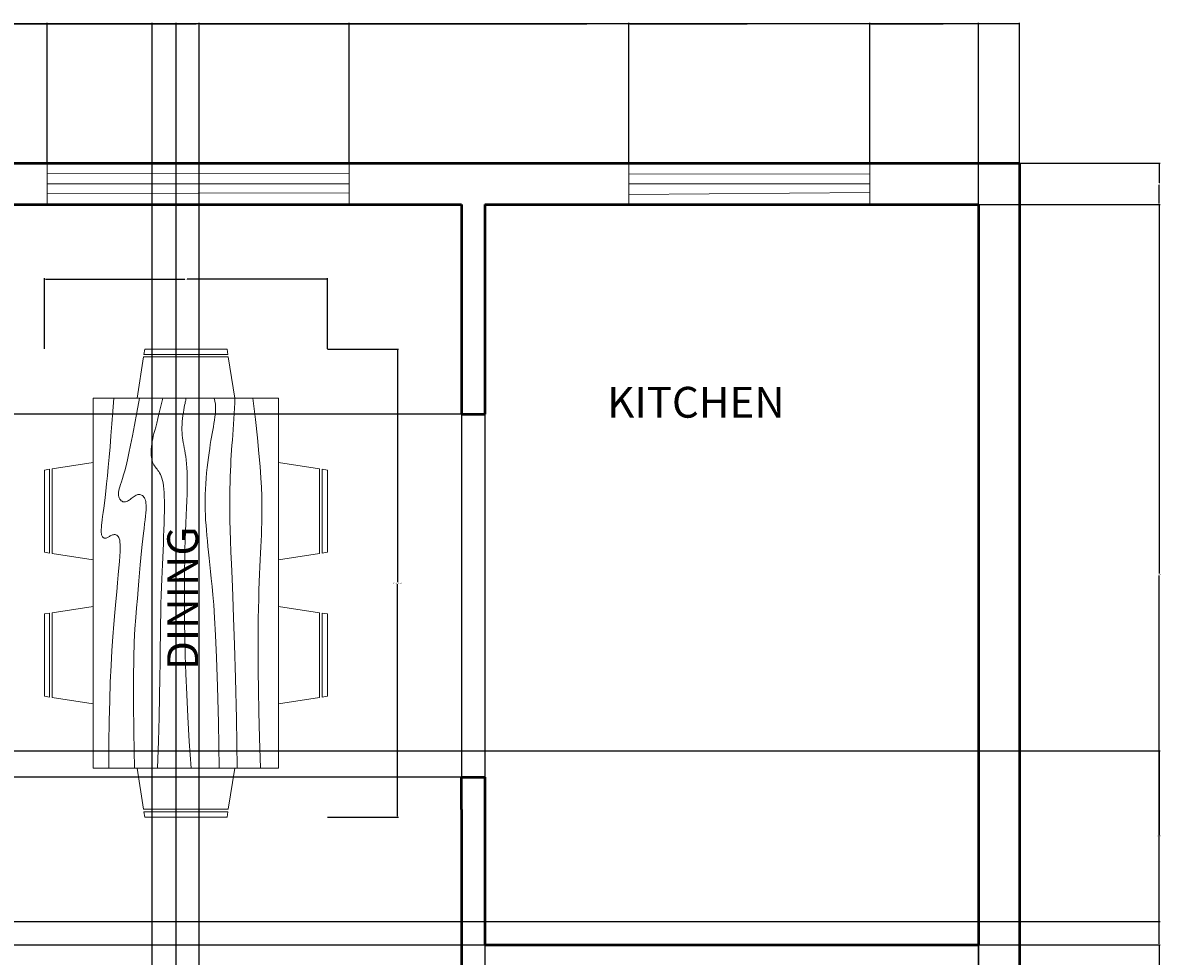
# Model space of a CAD drawing. Units: inches. Extents: x 2907 to 3328, y 1715 to 2286.
# Tile 5 of 5: x 3107 to 3328, y 2105 to 2286. Entities that reach past the tile are written whole.
import ezdxf

# ---------------------------------------------------------------- set-up
doc = ezdxf.new("R2010")
doc.units = ezdxf.units.IN
for name, color, linetype, lineweight in [('A-ANNO-DIMS', 2, 'Continuous', 18), ('A-AREA-IDEN', 7, 'Continuous', 25), ('A-FURN', 8, 'Continuous', 18), ('A-GLAZ', 4, 'Continuous', 18), ('A-WALL', 7, 'Continuous', 50)]:
    doc.layers.add(name, color=color, linetype=linetype, lineweight=lineweight)
doc.styles.get("Standard").update_dxf_attribs({"font": 'arial.ttf'})
doc.dimstyles.get("Standard").update_dxf_attribs({"dimtxt": 0.18, "dimasz": 0.18, "dimexe": 0.18, "dimexo": 0.0625, "dimgap": 0.09, "dimtad": 0, "dimtih": 1, "dimtoh": 1, "dimdec": 4, "dimzin": 0, "dimdsep": 46, "dimtxsty": 'Standard', "dimcen": 0.09, "dimadec": 0, "dimazin": 0, "dimtfac": 1, "dimtdec": 4, "dimtofl": 0, "dimtmove": 0, "dimatfit": 3, "dimfxl": 1, "dimtolj": 1, "dimtzin": 0, "dimarcsym": 0})

# ---------------------------------------------------------------- blocks, each defined once
blk = doc.blocks.new('Dining Set - 36 x 72 in.')
for p, q in [((-22, 27.5), (-22.1562, 26.50042)), ((-22, 27.5), (-6, 27.5)), ((-5.8437, 26.49966), (-6, 27.5)), ((6, 27.5), (5.8438, 26.50042)), ((6, 27.5), (22, 27.5)), ((22.1563, 26.49966), (22, 27.5)), ((-22.2343, 26.00059), (-23.4847, 17.99762)), ((-22.2304, 26), (-5.7608, 26)), ((-5.8416, 26.5), (-22.1534, 26.5)), ((-4.5152, 17.99762), (-5.7655, 25.99926)), ((5.7657, 26.00059), (4.5153, 17.99762)), ((5.7696, 26), (22.2392, 26)), ((22.1584, 26.5), (5.8466, 26.5)), ((23.4848, 17.99762), (22.2345, 25.99926)), ((36, 18), (-36, 18)), ((-36, 18), (-36, -18)), ((36, -18), (36, 18)), ((-44.0006, 8.23428), (-35.9976, 9.48474)), ((44.0006, 8.23428), (35.9976, 9.48474)), ((-45.5, 8), (-44.5004, 8.15617)), ((-45.5, 8), (-45.5, -8)), ((-44.5, -8.15843), (-44.5, 8.15338)), ((-44, 8.23041), (-44, -8.23915)), ((44, 8.23041), (44, -8.23915)), ((44.5, -8.15843), (44.5, 8.15338)), ((45.5, 8), (44.5005, 8.15617)), ((45.5, 8), (45.5, -8)), ((-44.4997, -8.15631), (-45.5, -8)), ((-35.9976, -9.48476), (-43.9993, -8.2345)), ((35.9976, -9.48476), (43.9993, -8.2345)), ((44.4997, -8.15631), (45.5, -8)), ((-36, -18), (36, -18)), ((-22.2343, -26.0006), (-23.4847, -17.99762)), ((-4.5152, -17.99762), (-5.7655, -25.99928)), ((5.7657, -26.0006), (4.5153, -17.99762)), ((23.4848, -17.99762), (22.2345, -25.99928)), ((-22.2304, -26), (-5.7608, -26)), ((-22, -27.5), (-22.1562, -26.50044)), ((-5.8416, -26.5), (-22.1534, -26.5)), ((-5.8437, -26.49967), (-6, -27.5)), ((5.7696, -26), (22.2392, -26)), ((6, -27.5), (5.8438, -26.50044)), ((22.1584, -26.5), (5.8466, -26.5)), ((22.1563, -26.49967), (22, -27.5)), ((-22, -27.5), (-6, -27.5)), ((6, -27.5), (22, -27.5))]:
    blk.add_line(p, q)
for points in [[(-36, 15), (-31.1772, 14.97754), (-26.8079, 14.91406), (-22.8538, 14.81543), (-19.276, 14.6875), (-16.0362, 14.53613), (-13.0957, 14.36718), (-10.4159, 14.18652), (-7.9583, 14), (-5.6904, 13.81315), (-3.6035, 13.63021), (-1.6954, 13.45508), (0.0365, 13.29166), (1.5945, 13.14388), (2.9811, 13.01562), (4.1988, 12.9108), (5.25, 12.83333), (6.1393, 12.78613), (6.8802, 12.76823), (7.4883, 12.77767), (7.9792, 12.8125), (8.3685, 12.87077), (8.6719, 12.95052), (8.9049, 13.0498), (9.0833, 13.16666), (9.2205, 13.29899), (9.3216, 13.44401), (9.3895, 13.59879), (9.4271, 13.76041), (9.4373, 13.92594), (9.4232, 14.09245), (9.3875, 14.257), (9.3333, 14.41666), (9.2638, 14.56917), (9.1836, 14.71484), (9.0975, 14.85465), (9.0104, 14.98958), (8.9272, 15.1206), (8.8529, 15.2487), (8.7922, 15.37483), (8.75, 15.5), (8.7305, 15.62467), (8.7344, 15.74739), (8.7617, 15.86621), (8.8125, 15.97916), (8.8867, 16.08431), (8.9844, 16.17968), (9.1055, 16.26334), (9.25, 16.33333), (9.4189, 16.38802), (9.6172, 16.42708), (9.8506, 16.45052), (10.125, 16.45833), (10.4463, 16.45052), (10.8203, 16.42708), (11.2529, 16.38802), (11.75, 16.33333), (12.3184, 16.26318), (12.9694, 16.17838), (13.7151, 16.07991), (14.5677, 15.96875), (15.5395, 15.84586), (16.6426, 15.71224), (17.8893, 15.56884), (19.2917, 15.41666), (20.859, 15.25667), (22.5879, 15.08984), (24.4721, 14.91715), (26.5052, 14.73958), (28.6809, 14.5581), (30.9929, 14.3737), (33.4347, 14.18733), (36, 14)], [(-36, 10), (-28.9766, 10.14274), (-23.1725, 10.20442), (-18.4241, 10.19775), (-14.5677, 10.13541), (-11.4399, 10.03011), (-8.877, 9.89453), (-6.7154, 9.74137), (-4.7917, 9.58333), (-2.9698, 9.43082), (-1.2246, 9.28515), (0.4415, 9.14534), (2.026, 9.01041), (3.5266, 8.87939), (4.9408, 8.7513), (6.266, 8.62516), (7.5, 8.5), (8.6411, 8.37549), (9.6914, 8.2539), (10.6538, 8.13818), (11.5312, 8.03125), (12.3267, 7.93603), (13.043, 7.85547), (13.6831, 7.79248), (14.25, 7.75), (14.7471, 7.7303), (15.1797, 7.73307), (15.5537, 7.75732), (15.875, 7.80208), (16.1494, 7.86637), (16.3828, 7.94922), (16.5811, 8.04964), (16.75, 8.16666), (16.8944, 8.29915), (17.0143, 8.44531), (17.1089, 8.60319), (17.1771, 8.77083), (17.218, 8.94629), (17.2305, 9.1276), (17.2137, 9.31282), (17.1667, 9.5), (17.0895, 9.6875), (16.987, 9.875), (16.8649, 10.0625), (16.7292, 10.25), (16.5856, 10.4375), (16.4401, 10.625), (16.2985, 10.8125), (16.1667, 11), (16.05, 11.18733), (15.9518, 11.3737), (15.8752, 11.5581), (15.8229, 11.73958), (15.798, 11.91715), (15.8034, 12.08984), (15.842, 12.25667), (15.9167, 12.41666), (16.0295, 12.56836), (16.1784, 12.70833), (16.3605, 12.83268), (16.5729, 12.9375), (16.8127, 13.01888), (17.0768, 13.07291), (17.3625, 13.0957), (17.6667, 13.08333), (17.9894, 13.03312), (18.3418, 12.94726), (18.7382, 12.82918), (19.1927, 12.68229), (19.7195, 12.51001), (20.3327, 12.31575), (21.0465, 12.10294), (21.875, 11.875), (22.8357, 11.63354), (23.959, 11.37304), (25.2786, 11.08618), (26.8282, 10.76562), (28.6414, 10.40405), (30.752, 9.99414), (33.1936, 9.52856), (36, 9)], [(-36, 5.5), (-30.7157, 5.3348), (-26.069, 5.20963), (-21.9946, 5.11767), (-18.4271, 5.05208), (-15.3009, 5.00602), (-12.5508, 4.97265), (-10.1112, 4.94515), (-7.9167, 4.91666), (-5.909, 4.88167), (-4.0586, 4.83984), (-2.3429, 4.79215), (-0.7396, 4.73958), (0.7739, 4.6831), (2.22, 4.6237), (3.6213, 4.56233), (5, 4.5), (6.373, 4.43782), (7.7344, 4.3776), (9.0723, 4.32129), (10.375, 4.27083), (11.6309, 4.22819), (12.8281, 4.19531), (13.9551, 4.17415), (15, 4.16666), (15.954, 4.17448), (16.819, 4.19791), (17.6001, 4.23698), (18.3021, 4.29166), (18.9299, 4.36198), (19.4883, 4.44791), (19.9823, 4.54948), (20.4167, 4.66666), (20.7969, 4.79899), (21.1302, 4.94401), (21.4245, 5.09879), (21.6875, 5.26041), (21.9271, 5.42594), (22.1511, 5.59245), (22.3672, 5.757), (22.5834, 5.91666), (22.8065, 6.06868), (23.0404, 6.21093), (23.2879, 6.34147), (23.5521, 6.45833), (23.8358, 6.55957), (24.142, 6.64323), (24.4735, 6.70735), (24.8334, 6.75), (25.2235, 6.76969), (25.642, 6.76692), (26.0858, 6.74267), (26.5521, 6.69791), (27.0379, 6.63362), (27.5404, 6.55078), (28.0565, 6.45036), (28.5834, 6.33333), (29.1242, 6.19987), (29.7071, 6.04687), (30.3661, 5.87044), (31.1354, 5.66666), (32.0493, 5.43164), (33.142, 5.16146), (34.4475, 4.85221), (36, 4.5)], [(-36, -1), (-30.7915, -0.6591), (-26.0195, -0.38216), (-21.6519, -0.16284), (-17.6563, 0.00521), (-14.0005, 0.12833), (-10.6523, 0.21289), (-7.5796, 0.26522), (-4.75, 0.29166), (-2.134, 0.29793), (0.2878, 0.28711), (2.5317, 0.26163), (4.6146, 0.22396), (6.5529, 0.17651), (8.3633, 0.12174), (10.0623, 0.06209), (11.6667, 0), (13.1899, -0.06201), (14.6341, -0.1211), (15.9982, -0.17432), (17.2813, -0.21875), (18.4823, -0.25147), (19.6003, -0.26953), (20.6343, -0.27002), (21.5834, -0.25), (22.4481, -0.20768), (23.2357, -0.14584), (23.9549, -0.06836), (24.6146, 0.02083), (25.2235, 0.11784), (25.7904, 0.21875), (26.3241, 0.31966), (26.8334, 0.41666), (27.3265, 0.50618), (27.8099, 0.58593), (28.2894, 0.65397), (28.7709, 0.70833), (29.2601, 0.74707), (29.763, 0.76823), (30.2855, 0.76985), (30.8334, 0.75), (31.4088, 0.70784), (31.9994, 0.64713), (32.589, 0.57275), (33.1615, 0.48958), (33.7008, 0.4025), (34.1908, 0.3164), (34.6153, 0.23616), (34.9584, 0.16666), (35.2099, 0.11165), (35.3848, 0.07031), (35.504, 0.04069), (35.5886, 0.02083), (35.6594, 0.00879), (35.7377, 0.0026), (35.8442, 0.00032), (36, 0)], [(-36, -6.5), (-27.1843, -6.31267), (-20.084, -6.1263), (-14.469, -5.9419), (-10.1094, -5.76042), (-6.7752, -5.58285), (-4.2363, -5.41016), (-2.2629, -5.24333), (-0.625, -5.08334), (0.8708, -4.93099), (2.2715, -4.78646), (3.5872, -4.64974), (4.8281, -4.52084), (6.0046, -4.39974), (7.127, -4.28646), (8.2053, -4.18099), (9.25, -4.08334), (10.2705, -3.99382), (11.2734, -3.91407), (12.2647, -3.84603), (13.25, -3.79167), (14.2354, -3.75293), (15.2266, -3.73177), (16.2295, -3.73015), (17.25, -3.75), (18.2912, -3.79248), (19.3451, -3.85547), (20.4009, -3.93604), (21.4479, -4.03125), (22.4754, -4.13819), (23.4727, -4.25391), (24.4289, -4.37549), (25.3334, -4.5), (26.1785, -4.62492), (26.9694, -4.74935), (27.7145, -4.87281), (28.4219, -4.99479), (29.1, -5.11483), (29.7572, -5.23242), (30.4016, -5.34709), (31.0417, -5.45834), (31.6837, -5.56437), (32.3262, -5.65821), (32.9658, -5.73153), (33.599, -5.77604), (34.2224, -5.78345), (34.8327, -5.74545), (35.4264, -5.65373), (36, -5.5)], [(-36, -10), (-26.4022, -9.81299), (-18.4675, -9.62891), (-11.9839, -9.45069), (-6.7396, -9.28125), (-2.5226, -9.12354), (0.8789, -8.98047), (3.6769, -8.85498), (6.0833, -8.75), (8.2767, -8.66765), (10.3021, -8.60677), (12.1712, -8.56543), (13.8958, -8.54167), (15.4876, -8.53353), (16.9583, -8.53907), (18.3197, -8.55632), (19.5834, -8.58334), (20.7616, -8.61841), (21.8685, -8.66081), (22.9188, -8.71004), (23.9271, -8.76563), (24.9081, -8.82707), (25.8763, -8.89388), (26.8465, -8.96558), (27.8334, -9.04167), (28.8474, -9.12118), (29.8828, -9.20117), (30.93, -9.27824), (31.9792, -9.34896), (33.0205, -9.40991), (34.0443, -9.45768), (35.0407, -9.48885), (36, -9.5)], [(-36, -14.5), (-30.0881, -14.33513), (-25.0332, -14.21224), (-20.7312, -14.12647), (-17.0781, -14.07292), (-13.97, -14.04671), (-11.3027, -14.04297), (-8.9724, -14.05681), (-6.875, -14.08334), (-4.9224, -14.11833), (-3.0905, -14.16016), (-1.3709, -14.20785), (0.2448, -14.26042), (1.7647, -14.3169), (3.1973, -14.3763), (4.5507, -14.43767), (5.8333, -14.5), (7.0554, -14.5621), (8.235, -14.62175), (9.3922, -14.67652), (10.5469, -14.72396), (11.7192, -14.76164), (12.929, -14.78711), (14.1965, -14.79794), (15.5417, -14.79167), (16.9933, -14.76424), (18.6152, -14.70508), (20.4804, -14.60197), (22.6615, -14.44271), (25.2312, -14.21509), (28.2624, -13.9069), (31.8277, -13.50594), (36, -13)]]:
    blk.add_lwpolyline(points)
blk = doc.blocks.new('*D9')
at = {"layer": 'A-ANNO-DIMS', "color": 0, "lineweight": -2, "transparency": 16777216}
for p, q in [((3166.06, 2222.66), (3179.83, 2222.66)), ((3179.65, 2222.48), (3179.65, 2177.34)), ((3179.65, 2131.84), (3179.65, 2176.98)), ((3166.06, 2131.66), (3179.83, 2131.66))]:
    blk.add_line(p, q, dxfattribs=at)
at = {"layer": 'A-ANNO-DIMS', "color": 0, "transparency": 16777216}
for points in [[(3179.62, 2222.48), (3179.68, 2222.48), (3179.65, 2222.66)], [(3179.62, 2131.84), (3179.68, 2131.84), (3179.65, 2131.66)]]:
    blk.add_solid(points, dxfattribs=at)
at = {"layer": 'Defpoints', "color": 0, "transparency": 16777216}
for p in [(3166, 2222.66), (3179.65, 2222.66), (3166, 2131.66)]:
    blk.add_point(p, dxfattribs=at)
at = {"layer": 'A-ANNO-DIMS', "color": 0, "transparency": 16777216, "insert": (3179.65, 2177.16), "char_height": 0.18, "attachment_point": 5}
blk.add_mtext('\\A1;DINING SET 91', dxfattribs=at)
blk = doc.blocks.new('*D10')
at = {"layer": 'A-ANNO-DIMS', "color": 0, "lineweight": -2, "transparency": 16777216}
for p, q in [((3111, 2222.72), (3111, 2236.49)), ((3111.18, 2236.31), (3138.28, 2236.31)), ((3165.82, 2236.31), (3138.72, 2236.31)), ((3166, 2222.72), (3166, 2236.49))]:
    blk.add_line(p, q, dxfattribs=at)
at = {"layer": 'A-ANNO-DIMS', "color": 0, "transparency": 16777216}
for points in [[(3111.18, 2236.34), (3111.18, 2236.28), (3111, 2236.31)], [(3165.82, 2236.34), (3165.82, 2236.28), (3166, 2236.31)]]:
    blk.add_solid(points, dxfattribs=at)
at = {"layer": 'Defpoints', "color": 0, "transparency": 16777216}
for p in [(3111, 2236.31), (3111, 2222.66), (3166, 2222.66)]:
    blk.add_point(p, dxfattribs=at)
at = {"layer": 'A-ANNO-DIMS', "color": 0, "transparency": 16777216, "insert": (3138.5, 2236.31), "char_height": 0.18, "attachment_point": 5}
blk.add_mtext('\\A1;55', dxfattribs=at)
blk = doc.blocks.new('*D13')
at = {"layer": 'A-ANNO-DIMS', "color": 0, "lineweight": -2, "transparency": 16777216}
for p, q in [((2934.59, 2258.89), (2934.59, 2286.16)), ((2934.77, 2285.98), (3117.3, 2285.98)), ((3300.41, 2285.98), (3117.88, 2285.98)), ((3300.59, 2258.89), (3300.59, 2286.16))]:
    blk.add_line(p, q, dxfattribs=at)
at = {"layer": 'A-ANNO-DIMS', "color": 0, "transparency": 16777216}
for points in [[(2934.77, 2286.01), (2934.77, 2285.95), (2934.59, 2285.98)], [(3300.41, 2286.01), (3300.41, 2285.95), (3300.59, 2285.98)]]:
    blk.add_solid(points, dxfattribs=at)
at = {"layer": 'Defpoints', "color": 0, "transparency": 16777216}
for p in [(3300.59, 2285.98), (2934.59, 2258.83), (3300.59, 2258.83)]:
    blk.add_point(p, dxfattribs=at)
at = {"layer": 'A-ANNO-DIMS', "color": 0, "transparency": 16777216, "insert": (3117.59, 2285.98), "char_height": 0.18, "attachment_point": 5}
blk.add_mtext('\\A1;366', dxfattribs=at)
blk = doc.blocks.new('*D17')
at = {"layer": 'A-ANNO-DIMS', "color": 0, "lineweight": -2, "transparency": 16777216}
for p, q in [((3080.59, 2250.77), (3080.59, 1715.5)), ((3192.09, 2250.77), (3192.09, 1715.5)), ((3080.77, 1715.68), (3135.95, 1715.68)), ((3191.91, 1715.68), (3136.73, 1715.68))]:
    blk.add_line(p, q, dxfattribs=at)
at = {"layer": 'A-ANNO-DIMS', "color": 0, "transparency": 16777216}
for points in [[(3080.77, 1715.71), (3080.77, 1715.65), (3080.59, 1715.68)], [(3191.91, 1715.71), (3191.91, 1715.65), (3192.09, 1715.68)]]:
    blk.add_solid(points, dxfattribs=at)
at = {"layer": 'Defpoints', "color": 0, "transparency": 16777216}
for p in [(3080.59, 2250.83), (3192.09, 2250.83), (3192.09, 1715.68)]:
    blk.add_point(p, dxfattribs=at)
at = {"layer": 'A-ANNO-DIMS', "color": 0, "transparency": 16777216, "insert": (3136.34, 1715.68), "char_height": 0.18, "attachment_point": 5}
blk.add_mtext('\\A1;111.5', dxfattribs=at)
blk = doc.blocks.new('*D18')
at = {"layer": 'A-ANNO-DIMS', "color": 0, "lineweight": -2, "transparency": 16777216}
for p, q in [((3196.59, 2250.77), (3196.59, 1715.5)), ((3292.59, 2250.77), (3292.59, 1715.5)), ((3196.77, 1715.68), (3244.37, 1715.68)), ((3292.41, 1715.68), (3244.81, 1715.68))]:
    blk.add_line(p, q, dxfattribs=at)
at = {"layer": 'A-ANNO-DIMS', "color": 0, "transparency": 16777216}
for points in [[(3196.77, 1715.71), (3196.77, 1715.65), (3196.59, 1715.68)], [(3292.41, 1715.71), (3292.41, 1715.65), (3292.59, 1715.68)]]:
    blk.add_solid(points, dxfattribs=at)
at = {"layer": 'Defpoints', "color": 0, "transparency": 16777216}
for p in [(3196.59, 2250.83), (3292.59, 2250.83), (3292.59, 1715.68)]:
    blk.add_point(p, dxfattribs=at)
at = {"layer": 'A-ANNO-DIMS', "color": 0, "transparency": 16777216, "insert": (3244.59, 1715.68), "char_height": 0.18, "attachment_point": 5}
blk.add_mtext('\\A1;96', dxfattribs=at)
blk = doc.blocks.new('*D21')
at = {"layer": 'A-ANNO-DIMS', "color": 0, "lineweight": -2, "transparency": 16777216}
for p, q in [((3111.54, 2258.89), (3111.54, 2286.16)), ((3111.72, 2285.98), (3140.51, 2285.98)), ((3170.08, 2285.98), (3141.3, 2285.98)), ((3170.26, 2258.89), (3170.26, 2286.16))]:
    blk.add_line(p, q, dxfattribs=at)
at = {"layer": 'A-ANNO-DIMS', "color": 0, "transparency": 16777216}
for points in [[(3111.72, 2286.01), (3111.72, 2285.95), (3111.54, 2285.98)], [(3170.08, 2286.01), (3170.08, 2285.95), (3170.26, 2285.98)]]:
    blk.add_solid(points, dxfattribs=at)
at = {"layer": 'Defpoints', "color": 0, "transparency": 16777216}
for p in [(3170.26, 2285.98), (3111.54, 2258.83), (3170.26, 2258.83)]:
    blk.add_point(p, dxfattribs=at)
at = {"layer": 'A-ANNO-DIMS', "color": 0, "transparency": 16777216, "insert": (3140.9, 2285.98), "char_height": 0.18, "attachment_point": 5}
blk.add_mtext('\\A1;58.72', dxfattribs=at)
blk = doc.blocks.new('*D22')
at = {"layer": 'A-ANNO-DIMS', "color": 0, "lineweight": -2, "transparency": 16777216}
for p, q in [((3170.26, 2258.89), (3170.26, 2286.16)), ((3170.44, 2285.98), (3197.04, 2285.98)), ((3224.42, 2285.98), (3197.83, 2285.98)), ((3224.6, 2258.89), (3224.6, 2286.16))]:
    blk.add_line(p, q, dxfattribs=at)
at = {"layer": 'A-ANNO-DIMS', "color": 0, "transparency": 16777216}
for points in [[(3170.44, 2286.01), (3170.44, 2285.95), (3170.26, 2285.98)], [(3224.42, 2286.01), (3224.42, 2285.95), (3224.6, 2285.98)]]:
    blk.add_solid(points, dxfattribs=at)
at = {"layer": 'Defpoints', "color": 0, "transparency": 16777216}
for p in [(3224.6, 2285.98), (3170.26, 2258.83), (3224.6, 2258.83)]:
    blk.add_point(p, dxfattribs=at)
at = {"layer": 'A-ANNO-DIMS', "color": 0, "transparency": 16777216, "insert": (3197.43, 2285.98), "char_height": 0.18, "attachment_point": 5}
blk.add_mtext('\\A1;54.34', dxfattribs=at)
blk = doc.blocks.new('*D23')
at = {"layer": 'A-ANNO-DIMS', "color": 0, "lineweight": -2, "transparency": 16777216}
for p, q in [((3224.6, 2258.89), (3224.6, 2286.16)), ((3224.78, 2285.98), (3247.65, 2285.98)), ((3271.31, 2285.98), (3248.44, 2285.98)), ((3271.49, 2258.89), (3271.49, 2286.16))]:
    blk.add_line(p, q, dxfattribs=at)
at = {"layer": 'A-ANNO-DIMS', "color": 0, "transparency": 16777216}
for points in [[(3224.78, 2286.01), (3224.78, 2285.95), (3224.6, 2285.98)], [(3271.31, 2286.01), (3271.31, 2285.95), (3271.49, 2285.98)]]:
    blk.add_solid(points, dxfattribs=at)
at = {"layer": 'Defpoints', "color": 0, "transparency": 16777216}
for p in [(3271.49, 2285.98), (3224.6, 2258.83), (3271.49, 2258.83)]:
    blk.add_point(p, dxfattribs=at)
at = {"layer": 'A-ANNO-DIMS', "color": 0, "transparency": 16777216, "insert": (3248.05, 2285.98), "char_height": 0.18, "attachment_point": 5}
blk.add_mtext('\\A1;46.89', dxfattribs=at)
blk = doc.blocks.new('*D24')
at = {"layer": 'A-ANNO-DIMS', "color": 0, "lineweight": -2, "transparency": 16777216}
for p, q in [((3271.49, 2258.89), (3271.49, 2286.16)), ((3271.67, 2285.98), (3285.73, 2285.98)), ((3300.41, 2285.98), (3286.35, 2285.98)), ((3300.59, 2258.89), (3300.59, 2286.16))]:
    blk.add_line(p, q, dxfattribs=at)
at = {"layer": 'A-ANNO-DIMS', "color": 0, "transparency": 16777216}
for points in [[(3271.67, 2286.01), (3271.67, 2285.95), (3271.49, 2285.98)], [(3300.41, 2286.01), (3300.41, 2285.95), (3300.59, 2285.98)]]:
    blk.add_solid(points, dxfattribs=at)
at = {"layer": 'Defpoints', "color": 0, "transparency": 16777216}
for p in [(3300.59, 2285.98), (3271.49, 2258.83), (3300.59, 2258.83)]:
    blk.add_point(p, dxfattribs=at)
at = {"layer": 'A-ANNO-DIMS', "color": 0, "transparency": 16777216, "insert": (3286.04, 2285.98), "char_height": 0.18, "attachment_point": 5}
blk.add_mtext('\\A1;29.1', dxfattribs=at)
blk = doc.blocks.new('*D28')
at = {"layer": 'A-ANNO-DIMS', "color": 0, "lineweight": -2, "transparency": 16777216}
for p, q in [((3292.65, 2250.83), (3327.92, 2250.83)), ((3327.74, 2250.65), (3327.74, 2179.01)), ((3327.74, 2107.01), (3327.74, 2178.65)), ((3292.65, 2106.83), (3327.92, 2106.83))]:
    blk.add_line(p, q, dxfattribs=at)
at = {"layer": 'A-ANNO-DIMS', "color": 0, "transparency": 16777216}
for points in [[(3327.71, 2250.65), (3327.77, 2250.65), (3327.74, 2250.83)], [(3327.71, 2107.01), (3327.77, 2107.01), (3327.74, 2106.83)]]:
    blk.add_solid(points, dxfattribs=at)
at = {"layer": 'Defpoints', "color": 0, "transparency": 16777216}
for p in [(3292.59, 2250.83), (3327.74, 2250.83), (3292.59, 2106.83)]:
    blk.add_point(p, dxfattribs=at)
at = {"layer": 'A-ANNO-DIMS', "color": 0, "transparency": 16777216, "insert": (3327.74, 2178.83), "char_height": 0.18, "attachment_point": 5}
blk.add_mtext('\\A1;144', dxfattribs=at)
blk = doc.blocks.new('*D32')
at = {"layer": 'A-ANNO-DIMS', "color": 0, "lineweight": -2, "transparency": 16777216}
for p, q in [((3141.09, 1786.89), (3141.09, 2286.16)), ((3141.27, 2285.98), (3216.45, 2285.98)), ((3292.41, 2285.98), (3217.23, 2285.98)), ((3292.59, 1786.89), (3292.59, 2286.16))]:
    blk.add_line(p, q, dxfattribs=at)
at = {"layer": 'A-ANNO-DIMS', "color": 0, "transparency": 16777216}
for points in [[(3141.27, 2286.01), (3141.27, 2285.95), (3141.09, 2285.98)], [(3292.41, 2286.01), (3292.41, 2285.95), (3292.59, 2285.98)]]:
    blk.add_solid(points, dxfattribs=at)
at = {"layer": 'Defpoints', "color": 0, "transparency": 16777216}
for p in [(3292.59, 2285.98), (3141.09, 1786.83), (3292.59, 1786.83)]:
    blk.add_point(p, dxfattribs=at)
at = {"layer": 'A-ANNO-DIMS', "color": 0, "transparency": 16777216, "insert": (3216.84, 2285.98), "char_height": 0.18, "attachment_point": 5}
blk.add_mtext('\\A1;151.5', dxfattribs=at)
blk = doc.blocks.new('*D34')
at = {"layer": 'A-ANNO-DIMS', "color": 0, "lineweight": -2, "transparency": 16777216}
for p, q in [((3074.5, 1778.89), (3074.5, 2286.16)), ((3074.68, 2285.98), (3102.84, 2285.98)), ((3131.79, 2285.98), (3103.63, 2285.98)), ((3131.97, 1778.89), (3131.97, 2286.16))]:
    blk.add_line(p, q, dxfattribs=at)
at = {"layer": 'A-ANNO-DIMS', "color": 0, "transparency": 16777216}
for points in [[(3074.68, 2286.01), (3074.68, 2285.95), (3074.5, 2285.98)], [(3131.79, 2286.01), (3131.79, 2285.95), (3131.97, 2285.98)]]:
    blk.add_solid(points, dxfattribs=at)
at = {"layer": 'Defpoints', "color": 0, "transparency": 16777216}
for p in [(3131.97, 2285.98), (3074.5, 1778.83), (3131.97, 1778.83)]:
    blk.add_point(p, dxfattribs=at)
at = {"layer": 'A-ANNO-DIMS', "color": 0, "transparency": 16777216, "insert": (3103.24, 2285.98), "char_height": 0.18, "attachment_point": 5}
blk.add_mtext('\\A1;57.47', dxfattribs=at)
blk = doc.blocks.new('*D37')
at = {"layer": 'A-ANNO-DIMS', "color": 0, "lineweight": -2, "transparency": 16777216}
for p, q in [((3076.15, 2144.51), (3327.92, 2144.51)), ((3327.74, 2144.33), (3327.74, 2128.1)), ((3327.74, 2111.51), (3327.74, 2127.74)), ((3080.65, 2111.33), (3327.92, 2111.33))]:
    blk.add_line(p, q, dxfattribs=at)
at = {"layer": 'A-ANNO-DIMS', "color": 0, "transparency": 16777216}
for points in [[(3327.71, 2144.33), (3327.77, 2144.33), (3327.74, 2144.51)], [(3327.71, 2111.51), (3327.77, 2111.51), (3327.74, 2111.33)]]:
    blk.add_solid(points, dxfattribs=at)
at = {"layer": 'Defpoints', "color": 0, "transparency": 16777216}
for p in [(3076.09, 2144.51), (3327.74, 2144.51), (3080.59, 2111.33)]:
    blk.add_point(p, dxfattribs=at)
at = {"layer": 'A-ANNO-DIMS', "color": 0, "transparency": 16777216, "insert": (3327.74, 2127.92), "char_height": 0.18, "attachment_point": 5}
blk.add_mtext('\\A1;33.185', dxfattribs=at)
blk = doc.blocks.new('*D39')
at = {"layer": 'A-ANNO-DIMS', "color": 0, "lineweight": -2, "transparency": 16777216}
for p, q in [((3076.15, 2106.83), (3327.92, 2106.83)), ((3327.74, 2106.65), (3327.74, 2091.21)), ((3327.74, 2075.41), (3327.74, 2090.85)), ((3080.65, 2075.23), (3327.92, 2075.23))]:
    blk.add_line(p, q, dxfattribs=at)
at = {"layer": 'A-ANNO-DIMS', "color": 0, "transparency": 16777216}
for points in [[(3327.71, 2106.65), (3327.77, 2106.65), (3327.74, 2106.83)], [(3327.71, 2075.41), (3327.77, 2075.41), (3327.74, 2075.23)]]:
    blk.add_solid(points, dxfattribs=at)
at = {"layer": 'Defpoints', "color": 0, "transparency": 16777216}
for p in [(3076.09, 2106.83), (3327.74, 2106.83), (3080.59, 2075.23)]:
    blk.add_point(p, dxfattribs=at)
at = {"layer": 'A-ANNO-DIMS', "color": 0, "transparency": 16777216, "insert": (3327.74, 2091.03), "char_height": 0.18, "attachment_point": 5}
blk.add_mtext('\\A1;31.604', dxfattribs=at)
blk = doc.blocks.new('*D44')
at = {"layer": 'A-ANNO-DIMS', "color": 0, "lineweight": -2, "transparency": 16777216}
for p, q in [((3192.03, 2210.04), (2907.26, 2210.04)), ((2907.44, 2209.86), (2907.44, 2174.92)), ((2907.44, 2139.62), (2907.44, 2174.56)), ((3192.03, 2139.44), (2907.26, 2139.44))]:
    blk.add_line(p, q, dxfattribs=at)
at = {"layer": 'A-ANNO-DIMS', "color": 0, "transparency": 16777216}
for points in [[(2907.41, 2209.86), (2907.47, 2209.86), (2907.44, 2210.04)], [(2907.41, 2139.62), (2907.47, 2139.62), (2907.44, 2139.44)]]:
    blk.add_solid(points, dxfattribs=at)
at = {"layer": 'Defpoints', "color": 0, "transparency": 16777216}
for p in [(2907.44, 2210.04), (3192.09, 2210.04), (3192.09, 2139.44)]:
    blk.add_point(p, dxfattribs=at)
at = {"layer": 'A-ANNO-DIMS', "color": 0, "transparency": 16777216, "insert": (2907.44, 2174.74), "char_height": 0.18, "attachment_point": 5}
blk.add_mtext('\\A1;70.6', dxfattribs=at)
blk = doc.blocks.new('*D45')
at = {"layer": 'A-ANNO-DIMS', "color": 0, "lineweight": -2, "transparency": 16777216}
for p, q in [((3192.03, 2250.83), (2907.26, 2250.83)), ((2907.44, 2250.65), (2907.44, 2230.62)), ((2907.44, 2210.22), (2907.44, 2230.25)), ((3192.03, 2210.04), (2907.26, 2210.04))]:
    blk.add_line(p, q, dxfattribs=at)
at = {"layer": 'A-ANNO-DIMS', "color": 0, "transparency": 16777216}
for points in [[(2907.41, 2250.65), (2907.47, 2250.65), (2907.44, 2250.83)], [(2907.41, 2210.22), (2907.47, 2210.22), (2907.44, 2210.04)]]:
    blk.add_solid(points, dxfattribs=at)
at = {"layer": 'Defpoints', "color": 0, "transparency": 16777216}
for p in [(2907.44, 2250.83), (3192.09, 2250.83), (3192.09, 2210.04)]:
    blk.add_point(p, dxfattribs=at)
at = {"layer": 'A-ANNO-DIMS', "color": 0, "transparency": 16777216, "insert": (2907.44, 2230.43), "char_height": 0.18, "attachment_point": 5}
blk.add_mtext('\\A1;40.79', dxfattribs=at)
blk = doc.blocks.new('*D46')
at = {"layer": 'A-ANNO-DIMS', "color": 0, "lineweight": -2, "transparency": 16777216}
for p, q in [((3300.65, 2258.83), (3327.92, 2258.83)), ((3327.74, 2258.65), (3327.74, 2255.01)), ((3327.74, 2251.01), (3327.74, 2254.65)), ((3292.65, 2250.83), (3327.92, 2250.83))]:
    blk.add_line(p, q, dxfattribs=at)
at = {"layer": 'A-ANNO-DIMS', "color": 0, "transparency": 16777216}
for points in [[(3327.71, 2258.65), (3327.77, 2258.65), (3327.74, 2258.83)], [(3327.71, 2251.01), (3327.77, 2251.01), (3327.74, 2250.83)]]:
    blk.add_solid(points, dxfattribs=at)
at = {"layer": 'Defpoints', "color": 0, "transparency": 16777216}
for p in [(3300.59, 2258.83), (3327.74, 2258.83), (3292.59, 2250.83)]:
    blk.add_point(p, dxfattribs=at)
at = {"layer": 'A-ANNO-DIMS', "color": 0, "transparency": 16777216, "insert": (3327.74, 2254.83), "char_height": 0.18, "attachment_point": 5}
blk.add_mtext('\\A1;8', dxfattribs=at)
blk = doc.blocks.new('*D56')
at = {"layer": 'A-ANNO-DIMS', "color": 0, "lineweight": -2, "transparency": 16777216}
for p, q in [((2942.59, 1786.89), (2942.59, 2286.16)), ((2942.77, 2285.98), (3039.31, 2285.98)), ((3136.41, 2285.98), (3039.87, 2285.98)), ((3136.59, 1786.89), (3136.59, 2286.16))]:
    blk.add_line(p, q, dxfattribs=at)
at = {"layer": 'A-ANNO-DIMS', "color": 0, "transparency": 16777216}
for points in [[(2942.77, 2286.01), (2942.77, 2285.95), (2942.59, 2285.98)], [(3136.41, 2286.01), (3136.41, 2285.95), (3136.59, 2285.98)]]:
    blk.add_solid(points, dxfattribs=at)
at = {"layer": 'Defpoints', "color": 0, "transparency": 16777216}
for p in [(3136.59, 2285.98), (2942.59, 1786.83), (3136.59, 1786.83)]:
    blk.add_point(p, dxfattribs=at)
at = {"layer": 'A-ANNO-DIMS', "color": 0, "transparency": 16777216, "insert": (3039.59, 2285.98), "char_height": 0.18, "attachment_point": 5}
blk.add_mtext('\\A1;194', dxfattribs=at)

msp = doc.modelspace()

# ---------------------------------------------------------------- linework, layer by layer
at = {"layer": 'A-GLAZ'}
for p, q in [((3111.5432, 2256.835), (3170.264, 2256.8975)), ((3224.6025, 2256.8033), (3271.4914, 2256.7345)), ((3111.5432, 2254.8301), (3170.264, 2254.8301)), ((3224.6025, 2254.8301), (3271.4914, 2254.8301)), ((3224.6025, 2252.7428), (3271.4914, 2253.1557)), ((3111.5432, 2252.9548), (3170.264, 2253.0832))]:
    msp.add_line(p, q, dxfattribs=at)
for points in [[(3111.5432, 2258.8301), (3170.264, 2258.8301), (3170.264, 2250.8301), (3111.5432, 2250.8301)], [(3224.6025, 2258.8301), (3271.4914, 2258.8301), (3271.4914, 2250.8301), (3224.6025, 2250.8301)]]:
    msp.add_lwpolyline(points, close=True, dxfattribs=at)
at = {"layer": 'A-WALL'}
for p, q in [((2934.5892, 2258.8301), (3300.5892, 2258.8301)), ((3300.5892, 2258.8301), (3300.5892, 1778.8301)), ((3080.5892, 2250.8301), (3192.0892, 2250.8301)), ((3192.0892, 2250.8301), (3192.0892, 2210.0384)), ((3196.5892, 2250.8301), (3196.5892, 2210.0384)), ((3196.5892, 2250.8301), (3292.5892, 2250.8301)), ((3292.5892, 2250.8301), (3292.5892, 2106.8301)), ((3192.0892, 2210.0384), (3196.5892, 2210.0384)), ((3192.0892, 2133.1037), (3192.0892, 2139.4387)), ((3192.0892, 2139.4387), (3196.5892, 2139.4387)), ((3196.5892, 2139.4387), (3196.5892, 2133.1037)), ((3192.0892, 2133.1037), (3192.0892, 2106.8301)), ((3196.5892, 2133.1037), (3196.5892, 2106.8301)), ((3192.0892, 2106.8301), (3192.0892, 2102.3301)), ((3196.5892, 2106.8301), (3292.5892, 2106.8301))]:
    msp.add_line(p, q, dxfattribs=at)

# ---------------------------------------------------------------- block references
at = {"layer": 'A-FURN', "rotation": 90}
msp.add_blockref('Dining Set - 36 x 72 in.', (3138.5003, 2177.1584), dxfattribs=at)

# ---------------------------------------------------------------- texts
at = {"layer": 'A-AREA-IDEN', "insert": (3220.4055, 2215.3404), "char_height": 6, "attachment_point": 1}
msp.add_mtext_dynamic_manual_height_columns('KITCHEN', width=50.965346, gutter_width=12.5, heights=[0], dxfattribs=at)
at = {"layer": 'A-AREA-IDEN', "insert": (3134.8855, 2160.2514), "char_height": 6, "attachment_point": 1, "rotation": 90}
msp.add_mtext_dynamic_manual_height_columns('DINING ', width=50.965346, gutter_width=12.5, heights=[0], dxfattribs=at)

# ---------------------------------------------------------------- dimensions: what is measured, and where the dimension line sits
at = {"layer": 'A-ANNO-DIMS'}
for base, p1, p2, override, picture, middle in [((3300.5892, 2285.9816), (2934.5892, 2258.8301), (3300.5892, 2258.8301), {"dimdec": 0, "dimlfac": 1, "dimrnd": 0, "dimzin": 0, "dimdsep": 46, "dimlunit": 2}, '*D13', (3117.5892, 2285.9816)), ((3136.5892, 2285.9816), (2942.5892, 1786.8301), (3136.5892, 1786.8301), {"dimdec": 0, "dimlfac": 1, "dimrnd": 0, "dimzin": 0, "dimdsep": 46, "dimlunit": 2}, '*D56', (3039.5892, 2285.9816)), ((3131.9734, 2285.9816), (3074.499, 1778.8301), (3131.9734, 1778.8301), {"dimdec": 2, "dimlfac": 1, "dimrnd": 0, "dimzin": 0, "dimdsep": 46, "dimlunit": 2}, '*D34', (3103.2362, 2285.9816)), ((3170.264, 2285.9816), (3111.5432, 2258.8301), (3170.264, 2258.8301), {"dimdec": 2, "dimlfac": 1, "dimrnd": 0, "dimzin": 0, "dimdsep": 46, "dimlunit": 2}, '*D21', (3140.9036, 2285.9816)), ((3292.5892, 2285.9816), (3141.0892, 1786.8301), (3292.5892, 1786.8301), {"dimdec": 1, "dimlfac": 1, "dimrnd": 0, "dimzin": 0, "dimdsep": 46, "dimlunit": 2}, '*D32', (3216.8392, 2285.9816)), ((3224.6025, 2285.9816), (3170.264, 2258.8301), (3224.6025, 2258.8301), {"dimdec": 2, "dimlfac": 1, "dimrnd": 0, "dimzin": 0, "dimdsep": 46, "dimlunit": 2}, '*D22', (3197.4332, 2285.9816)), ((3271.4914, 2285.9816), (3224.6025, 2258.8301), (3271.4914, 2258.8301), {"dimdec": 2, "dimlfac": 1, "dimrnd": 0, "dimzin": 0, "dimdsep": 46, "dimlunit": 2}, '*D23', (3248.0469, 2285.9816)), ((3300.5892, 2285.9816), (3271.4914, 2258.8301), (3300.5892, 2258.8301), {"dimdec": 1, "dimlfac": 1, "dimrnd": 0, "dimzin": 0, "dimdsep": 46, "dimlunit": 2}, '*D24', (3286.0403, 2285.9816)), ((3192.0892, 1715.6786), (3080.5892, 2250.8301), (3192.0892, 2250.8301), {"dimdec": 1, "dimlfac": 1, "dimrnd": 0, "dimzin": 0, "dimdsep": 46, "dimlunit": 2}, '*D17', (3136.3392, 1715.6786)), ((3292.5892, 1715.6786), (3196.5892, 2250.8301), (3292.5892, 2250.8301), {"dimdec": 0, "dimlfac": 1, "dimrnd": 0, "dimzin": 0, "dimdsep": 46, "dimlunit": 2}, '*D18', (3244.5892, 1715.6786))]:
    dim = msp.add_linear_dim(base=base, p1=p1, p2=p2, dimstyle='Standard', override=override, dxfattribs=at)
    dim.commit()
    dim.dimension.update_dxf_attribs({"geometry": picture, "text_midpoint": middle})
for base, p1, p2, angle, override, picture, middle in [((3327.7407, 2258.8301), (3292.5892, 2250.8301), (3300.5892, 2258.8301), 90, {"dimdec": 0, "dimlfac": 1, "dimrnd": 0, "dimzin": 0, "dimdsep": 46, "dimlunit": 2}, '*D46', (3327.7407, 2254.8301)), ((2907.4377, 2250.8301), (3192.0892, 2210.0384), (3192.0892, 2250.8301), 90, {"dimdec": 2, "dimlfac": 1, "dimrnd": 0, "dimzin": 0, "dimdsep": 46, "dimlunit": 2}, '*D45', (2907.4377, 2230.4342)), ((3327.7407, 2250.8301), (3292.5892, 2106.8301), (3292.5892, 2250.8301), 90, {"dimdec": 0, "dimlfac": 1, "dimrnd": 0, "dimzin": 0, "dimdsep": 46, "dimlunit": 2}, '*D28', (3327.7407, 2178.8301)), ((3111.0003, 2236.3084), (3166.0003, 2222.6584), (3111.0003, 2222.6584), 180, {"dimdec": 0, "dimlfac": 1, "dimrnd": 0, "dimzin": 0, "dimdsep": 46, "dimlunit": 2}, '*D10', (3138.5003, 2236.3084)), ((2907.4377, 2210.0384), (3192.0892, 2139.4387), (3192.0892, 2210.0384), 90, {"dimdec": 1, "dimlfac": 1, "dimrnd": 0, "dimzin": 0, "dimdsep": 46, "dimlunit": 2}, '*D44', (2907.4377, 2174.7386)), ((3327.7407, 2144.5149), (3080.5892, 2111.3301), (3076.0892, 2144.5149), 90, {"dimdec": 3, "dimlfac": 1, "dimrnd": 0, "dimzin": 0, "dimdsep": 46, "dimlunit": 2}, '*D37', (3327.7407, 2127.9225)), ((3327.7407, 2106.8301), (3080.5892, 2075.2259), (3076.0892, 2106.8301), 90, {"dimdec": 3, "dimlfac": 1, "dimrnd": 0, "dimzin": 0, "dimdsep": 46, "dimlunit": 2}, '*D39', (3327.7407, 2091.028))]:
    dim = msp.add_linear_dim(base=base, p1=p1, p2=p2, angle=angle, dimstyle='Standard', override=override, dxfattribs=at)
    dim.commit()
    dim.dimension.update_dxf_attribs({"geometry": picture, "text_midpoint": middle})
dim = msp.add_linear_dim(base=(3179.6503, 2222.6584), p1=(3166.0003, 2131.6584), p2=(3166.0003, 2222.6584), angle=90, text='DINING SET <>', dimstyle='Standard', override={"dimdec": 0, "dimlfac": 1, "dimrnd": 0, "dimzin": 0, "dimdsep": 46, "dimlunit": 2}, dxfattribs=at)
dim.commit()
dim.dimension.update_dxf_attribs({"geometry": '*D9', "text_midpoint": (3179.6503, 2177.1584)})

doc.saveas('drawing.dxf')
